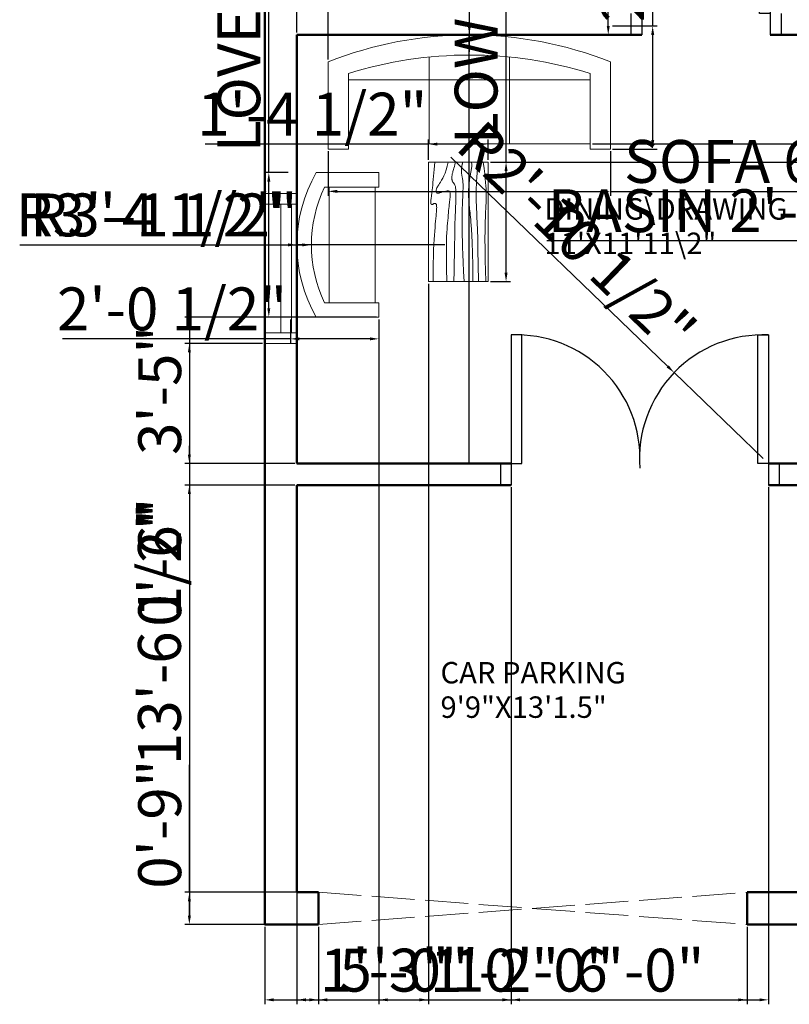
# Model space of a CAD drawing. Units: inches. Extents: x 3705 to 4206, y -1241 to -584.
# Tile 1 of 3: x 3705 to 3921, y -1162 to -886. Entities that reach past the tile are written whole.
import ezdxf

# ---------------------------------------------------------------- set-up
doc = ezdxf.new("R2010")
doc.units = ezdxf.units.IN
doc.linetypes.add('ACAD_ISO02W100', pattern=[15, 12, -3])
for name, color, linetype, lineweight in [('A-ANNO-DIMS', 2, 'Continuous', 18), ('A-AREA-IDEN', 7, 'Continuous', 25), ('A-DOOR', 3, 'Continuous', 25), ('A-DOOR-HIDN', 3, 'ACAD_ISO02W100', 18), ('A-FURN', 8, 'Continuous', 18), ('A-GLAZ', 4, 'Continuous', 18), ('A-WALL', 7, 'Continuous', 50)]:
    doc.layers.add(name, color=color, linetype=linetype, lineweight=lineweight)
doc.styles.get("Standard").update_dxf_attribs({"font": 'arial.ttf'})
doc.dimstyles.new('ISO-25', dxfattribs={"dimtxt": 12, "dimasz": 2.5, "dimexe": 1.25, "dimexo": 0.625, "dimtad": 1, "dimdec": 1, "dimlunit": 3, "dimtxsty": 'Standard', "dimcen": 2.5, "dimadec": 0, "dimazin": 0, "dimtfac": 1, "dimtdec": 1, "dimtmove": 0, "dimatfit": 3, "dimfxl": 1, "dimarcsym": 0})

# ---------------------------------------------------------------- blocks, each defined once
blk = doc.blocks.new('Sofa - Roundback Loveseat 5 ft.')
for p, q in [((0, -32.44198), (0, -5.99998)), ((-24, -33.99998), (-24, -11.46958)), ((24.00004, -33.99998), (24.00004, -11.46958)), ((-23.9998, -13.38178), (23.99986, -13.38178)), ((-24, -32.44198), (24.00004, -32.44198))]:
    blk.add_line(p, q)
for points in [[(-24, -33.99998), (-30, -33.99998), (-30, -7.99998)], [(30.00004, -7.99998), (30.00004, -33.99998), (24.00004, -33.99998)]]:
    blk.add_lwpolyline(points)
for centre, radius, start, end in [((0, -60.24998), 60.24998, 60.13715, 119.8628), ((0, -61.38438), 55.38444, 64.32083, 115.6792)]:
    blk.add_arc(centre, radius, start, end)
blk = doc.blocks.new('Sofa - Roundback 7 ft.')
for p, q in [((-12.00002, -32.4421), (-12.00003, -6.5971)), ((11.99997, -32.4421), (11.99998, -6.5971)), ((-36.000027, -34), (-36.000027, -11.4696)), ((35.99998, -34), (35.99998, -11.4696)), ((-35.999844, -13.3819), (35.9998, -13.3819)), ((-36.000027, -32.4421), (35.99998, -32.4421))]:
    blk.add_line(p, q)
for points in [[(-36.000027, -34), (-42.000027, -34), (-42.000027, -8)], [(41.99998, -8), (41.99998, -34), (35.99998, -34)]]:
    blk.add_lwpolyline(points)
for centre, radius, start, end in [((0, -114.25), 114.25, 68.43141, 111.5686), ((-0.00001, -127.1968), 121.1968, 72.72033, 107.2797)]:
    blk.add_arc(centre, radius, start, end)
blk = doc.blocks.new('Table - Rectangular Woodgrain 60 x 30 in.')
for p, q in [((0, 0), (0, -30)), ((60, 0), (0, 0)), ((60, -30), (60, 0)), ((0, -30), (60, -30))]:
    blk.add_line(p, q)
for points in [[(0, -2.4), (4.8155, -2.418), (9.0302, -2.4688), (12.709, -2.5477), (15.9167, -2.65), (18.7181, -2.7711), (21.1781, -2.9063), (23.3616, -3.0508), (25.3333, -3.2), (27.1477, -3.3495), (28.8172, -3.4958), (30.3437, -3.636), (31.7291, -3.7667), (32.9756, -3.8849), (34.0849, -3.9875), (35.059, -4.0714), (35.9, -4.1334), (36.6114, -4.1711), (37.2041, -4.1854), (37.6906, -4.1779), (38.0833, -4.15), (38.3948, -4.1034), (38.6375, -4.0396), (38.8239, -3.9602), (38.9666, -3.8667), (39.0764, -3.7608), (39.1573, -3.6448), (39.2116, -3.521), (39.2416, -3.3917), (39.2498, -3.2593), (39.2385, -3.1261), (39.21, -2.9944), (39.1666, -2.8667), (39.111, -2.7447), (39.0468, -2.6281), (38.978, -2.5163), (38.9083, -2.4083), (38.8418, -2.3035), (38.7823, -2.201), (38.7337, -2.1001), (38.7, -2), (38.6844, -1.9003), (38.6875, -1.8021), (38.7094, -1.707), (38.75, -1.6167), (38.8094, -1.5326), (38.8875, -1.4563), (38.9844, -1.3893), (39.1, -1.3333), (39.2351, -1.2896), (39.3937, -1.2583), (39.5804, -1.2396), (39.8, -1.2333), (40.057, -1.2396), (40.3562, -1.2583), (40.7023, -1.2896), (41.1, -1.3333), (41.5547, -1.3895), (42.0755, -1.4573), (42.6721, -1.5361), (43.3542, -1.625), (44.1316, -1.7233), (45.014, -1.8302), (46.0114, -1.9449), (47.1333, -2.0667), (48.3862, -2.1947), (49.7625, -2.3281), (51.2513, -2.4663), (52.8416, -2.6083), (54.5226, -2.7535), (56.2833, -2.9011), (58.1127, -3.0501), (60, -3.2)], [(0, -9.2), (6.5759, -9.0858), (11.9385, -9.0365), (16.2527, -9.0418), (19.6833, -9.0917), (22.3952, -9.1759), (24.5531, -9.2844), (26.322, -9.4069), (27.8666, -9.5333), (29.3241, -9.6553), (30.7203, -9.7719), (32.0532, -9.8837), (33.3208, -9.9917), (34.5213, -10.0965), (35.6526, -10.199), (36.7128, -10.2999), (37.7, -10.4), (38.6129, -10.4996), (39.4531, -10.5969), (40.223, -10.6895), (40.925, -10.775), (41.5613, -10.8512), (42.1344, -10.9156), (42.6465, -10.966), (43.1, -11), (43.4976, -11.0158), (43.8437, -11.0136), (44.143, -10.9942), (44.4, -10.9583), (44.6195, -10.9069), (44.8062, -10.8406), (44.9648, -10.7603), (45.1, -10.6667), (45.2155, -10.5598), (45.3114, -10.4365), (45.3871, -10.2929), (45.4416, -10.125), (45.4743, -9.929), (45.4844, -9.7011), (45.4709, -9.4371), (45.4333, -9.1333), (45.3716, -8.7883), (45.2896, -8.4104), (45.1919, -8.0107), (45.0833, -7.6), (44.9685, -7.1893), (44.8521, -6.7896), (44.7388, -6.4117), (44.6333, -6.0667), (44.54, -5.7628), (44.4614, -5.4979), (44.4001, -5.2675), (44.3583, -5.0667), (44.3384, -4.8909), (44.3427, -4.7354), (44.3736, -4.5956), (44.4333, -4.4667), (44.5236, -4.3453), (44.6427, -4.2333), (44.7884, -4.1339), (44.9583, -4.05), (45.1501, -3.9849), (45.3614, -3.9417), (45.59, -3.9234), (45.8333, -3.9333), (46.0915, -3.9749), (46.3734, -4.0531), (46.6906, -4.1736), (47.0542, -4.3417), (47.4756, -4.5629), (47.9661, -4.8427), (48.5372, -5.1866), (49.2, -5.6), (49.9676, -6.0844), (50.8594, -6.625), (51.8965, -7.2031), (53.1, -7.8), (54.491, -8.3969), (56.0906, -8.975), (57.9199, -9.5156), (60, -10)], [(0, -12.8), (5.1847, -12.9322), (9.6213, -13.0323), (13.3963, -13.1059), (16.5958, -13.1583), (19.3063, -13.1952), (21.614, -13.2219), (23.6054, -13.2439), (25.3666, -13.2667), (26.9728, -13.2947), (28.4531, -13.3281), (29.8256, -13.3663), (31.1083, -13.4083), (32.3191, -13.4535), (33.476, -13.501), (34.597, -13.5501), (35.7, -13.6), (36.7984, -13.6497), (37.8875, -13.6979), (38.9578, -13.743), (40, -13.7833), (41.0047, -13.8174), (41.9625, -13.8438), (42.864, -13.8607), (43.7, -13.8667), (44.4631, -13.8604), (45.1552, -13.8417), (45.7801, -13.8104), (46.3416, -13.7667), (46.8439, -13.7104), (47.2906, -13.6417), (47.6858, -13.5604), (48.0333, -13.4667), (48.3375, -13.3608), (48.6042, -13.2448), (48.8396, -13.121), (49.05, -12.9917), (49.2417, -12.8593), (49.4208, -12.7261), (49.5937, -12.5944), (49.7667, -12.4667), (49.9452, -12.3451), (50.1323, -12.2313), (50.3303, -12.1268), (50.5416, -12.0333), (50.7686, -11.9524), (51.0135, -11.8854), (51.2788, -11.8341), (51.5666, -11.8), (51.8785, -11.7843), (52.2116, -11.7865), (52.562, -11.8059), (52.926, -11.8417), (53.2998, -11.8931), (53.6795, -11.9594), (54.0614, -12.0397), (54.4416, -12.1333), (54.8223, -12.2401), (55.2293, -12.3625), (55.6942, -12.5037), (56.2489, -12.6667), (56.9251, -12.8547), (57.7545, -13.0708), (58.7689, -13.3182), (60, -13.6)], [(0, -18), (5.124, -17.7273), (9.6609, -17.5057), (13.6705, -17.3303), (17.2125, -17.1958), (20.3467, -17.0973), (23.1328, -17.0297), (25.6307, -16.9878), (27.9, -16.9667), (29.9928, -16.9617), (31.9302, -16.9703), (33.7254, -16.9907), (35.3917, -17.0208), (36.9423, -17.0588), (38.3906, -17.1026), (39.7499, -17.1503), (41.0333, -17.2), (42.2519, -17.2496), (43.4073, -17.2969), (44.4986, -17.3395), (45.525, -17.375), (46.4858, -17.4012), (47.3802, -17.4156), (48.2074, -17.416), (48.9667, -17.4), (49.6583, -17.3662), (50.2872, -17.3167), (50.8595, -17.2547), (51.3812, -17.1833), (51.8584, -17.1057), (52.2971, -17.025), (52.7034, -16.9443), (53.0833, -16.8667), (53.443, -16.7951), (53.789, -16.7313), (54.128, -16.6768), (54.4666, -16.6334), (54.8115, -16.6024), (55.1693, -16.5854), (55.5465, -16.5841), (55.95, -16.6), (56.3828, -16.6337), (56.8346, -16.6823), (57.2915, -16.7418), (57.7396, -16.8084), (58.165, -16.878), (58.5539, -16.9469), (58.8924, -17.0111), (59.1666, -17.0667), (59.3679, -17.1107), (59.5078, -17.1438), (59.6032, -17.1675), (59.6708, -17.1833), (59.7275, -17.193), (59.7901, -17.1979), (59.8753, -17.1998), (60, -17.2)], [(0, -22.4), (8.0098, -22.2501), (14.4094, -22.1011), (19.4168, -21.9535), (23.25, -21.8083), (26.1269, -21.6663), (28.2656, -21.5281), (29.884, -21.3947), (31.2, -21.2667), (32.3967, -21.1448), (33.5172, -21.0292), (34.5697, -20.9198), (35.5625, -20.8167), (36.5037, -20.7198), (37.4015, -20.6292), (38.2642, -20.5448), (39.1, -20.4667), (39.9164, -20.3951), (40.7187, -20.3313), (41.5117, -20.2768), (42.3, -20.2333), (43.0883, -20.2024), (43.8812, -20.1854), (44.6836, -20.1841), (45.5, -20.2), (46.3328, -20.234), (47.1747, -20.2844), (48.0163, -20.3488), (48.8479, -20.425), (49.66, -20.5106), (50.4429, -20.6031), (51.1872, -20.7004), (51.8833, -20.8), (52.5246, -20.8999), (53.1166, -20.9995), (53.6681, -21.0983), (54.1875, -21.1958), (54.6834, -21.2919), (55.1646, -21.3859), (55.6394, -21.4777), (56.1167, -21.5667), (56.6028, -21.6515), (57.0961, -21.7266), (57.5929, -21.7852), (58.0896, -21.8208), (58.5823, -21.8268), (59.0674, -21.7964), (59.5412, -21.723), (60, -21.6)], [(0, -25.2), (8.6355, -25.0504), (15.7026, -24.9031), (21.4049, -24.7606), (25.9458, -24.625), (29.529, -24.4988), (32.3578, -24.3844), (34.6359, -24.284), (36.5667, -24.2), (38.3213, -24.1341), (39.9417, -24.0854), (41.437, -24.0523), (42.8167, -24.0333), (44.0901, -24.0268), (45.2667, -24.0313), (46.3557, -24.0451), (47.3667, -24.0667), (48.309, -24.0947), (49.1928, -24.1287), (50.0284, -24.168), (50.826, -24.2125), (51.5959, -24.2617), (52.3483, -24.3151), (53.0935, -24.3725), (53.8417, -24.4334), (54.6009, -24.497), (55.3699, -24.561), (56.1454, -24.6226), (56.9239, -24.6792), (57.7021, -24.7279), (58.4764, -24.7662), (59.2435, -24.7911), (60, -24.8)], [(0, -28.8), (5.6867, -28.6681), (10.45, -28.5698), (14.407, -28.5012), (17.675, -28.4584), (20.3711, -28.4374), (22.6125, -28.4344), (24.5164, -28.4455), (26.2, -28.4667), (27.762, -28.4947), (29.2276, -28.5281), (30.6033, -28.5663), (31.8958, -28.6084), (33.1118, -28.6535), (34.2578, -28.7011), (35.3405, -28.7501), (36.3666, -28.8), (37.3443, -28.8497), (38.288, -28.8974), (39.2137, -28.9412), (40.1375, -28.9792), (41.0753, -29.0093), (42.0432, -29.0297), (43.0572, -29.0384), (44.1333, -29.0333), (45.2936, -29.0114), (46.5843, -28.9641), (48.0579, -28.8816), (49.7666, -28.7542), (51.7629, -28.5721), (54.0989, -28.3255), (56.8272, -28.0048), (60, -27.6)]]:
    blk.add_lwpolyline(points)
blk = doc.blocks.new('DOOR-SINGLE-36IN')
for p, q in [((0, 6), (0, 0)), ((3, 6), (3, 0)), ((39, 6), (39, 0)), ((42, 6), (42, 0))]:
    blk.add_line(p, q)
blk.add_lwpolyline([(39, 6), (36, 6), (36, 42), (39, 42)], close=True)
blk.add_arc((37.5, 7.5), 34.53, 87.5104, 182.4896)
blk = doc.blocks.new('WIN-SASH-36IN')
for p, q in [((0, 9), (0, 0)), ((36, 0), (36, 9)), ((0, 4.5), (36, 4.5)), ((0, 1.5), (36, 1.5)), ((0, 1.5), (36, 1.5))]:
    blk.add_line(p, q)
blk = doc.blocks.new('*D21')
at = {"layer": 'A-ANNO-DIMS', "color": 0, "lineweight": -2, "transparency": 16777216}
for p, q in [((3870.22, -848.33), (3870.22, -651.86)), ((3875.95, -848.33), (3868.97, -848.33)), ((3870.22, -888.25), (3870.22, -850.83)), ((3875.95, -890.75), (3868.97, -890.75))]:
    blk.add_line(p, q, dxfattribs=at)
at = {"layer": 'A-ANNO-DIMS', "color": 0, "transparency": 16777216}
for points in [[(3869.8, -850.83), (3870.63, -850.83), (3870.22, -848.33)], [(3869.8, -888.25), (3870.63, -888.25), (3870.22, -890.75)]]:
    blk.add_solid(points, dxfattribs=at)
at = {"layer": 'Defpoints', "color": 0, "transparency": 16777216}
for p in [(3870.22, -848.33), (3876.58, -848.33), (3876.58, -890.75)]:
    blk.add_point(p, dxfattribs=at)
at = {"layer": 'A-ANNO-DIMS', "color": 0, "transparency": 16777216, "insert": (3863.38, -748.84), "char_height": 12, "attachment_point": 5, "rotation": 90}
blk.add_mtext('DOOR SET 3\'-6 1/2" TYP.', dxfattribs=at)
blk = doc.blocks.new('*D23')
at = {"layer": 'A-ANNO-DIMS', "color": 0, "lineweight": -2, "transparency": 16777216}
for p, q in [((3775.21, -929.3), (3775.21, -773.05)), ((3780.66, -929.3), (3773.96, -929.3)), ((3775.21, -967.26), (3775.21, -931.8)), ((3780.66, -969.76), (3773.96, -969.76))]:
    blk.add_line(p, q, dxfattribs=at)
at = {"layer": 'A-ANNO-DIMS', "color": 0, "transparency": 16777216}
for points in [[(3774.79, -931.8), (3775.63, -931.8), (3775.21, -929.3)], [(3774.79, -967.26), (3775.63, -967.26), (3775.21, -969.76)]]:
    blk.add_solid(points, dxfattribs=at)
at = {"layer": 'Defpoints', "color": 0, "transparency": 16777216}
for p in [(3775.21, -929.3), (3781.28, -929.3), (3781.28, -969.76)]:
    blk.add_point(p, dxfattribs=at)
at = {"layer": 'A-ANNO-DIMS', "color": 0, "transparency": 16777216, "insert": (3768.37, -849.92), "char_height": 12, "attachment_point": 5, "rotation": 90}
blk.add_mtext('LOVESEAT 3\'-4 1/2"', dxfattribs=at)
blk = doc.blocks.new('*D24')
at = {"layer": 'A-ANNO-DIMS', "color": 0, "lineweight": -2, "transparency": 16777216}
for p, q in [((3781.28, -970.39), (3781.28, -977.08)), ((3806.01, -970.39), (3806.01, -977.08)), ((3781.28, -975.83), (3717.47, -975.83)), ((3803.51, -975.83), (3783.78, -975.83))]:
    blk.add_line(p, q, dxfattribs=at)
at = {"layer": 'A-ANNO-DIMS', "color": 0, "transparency": 16777216}
for points in [[(3783.78, -975.42), (3783.78, -976.25), (3781.28, -975.83)], [(3803.51, -975.42), (3803.51, -976.25), (3806.01, -975.83)]]:
    blk.add_solid(points, dxfattribs=at)
at = {"layer": 'Defpoints', "color": 0, "transparency": 16777216}
for p in [(3781.28, -969.76), (3806.01, -969.76), (3781.28, -975.83)]:
    blk.add_point(p, dxfattribs=at)
at = {"layer": 'A-ANNO-DIMS', "color": 0, "transparency": 16777216, "insert": (3748.12, -969), "char_height": 12, "attachment_point": 5}
blk.add_mtext('2\'-0 1/2"', dxfattribs=at)
blk = doc.blocks.new('*D25')
at = {"layer": 'A-ANNO-DIMS', "color": 0, "lineweight": -2, "transparency": 16777216}
for p, q in [((3791.85, -923.33), (3791.85, -935.8)), ((3870.81, -923.33), (3870.81, -935.8)), ((3794.35, -934.55), (3868.31, -934.55)), ((3870.81, -934.55), (3956.7, -934.55))]:
    blk.add_line(p, q, dxfattribs=at)
at = {"layer": 'A-ANNO-DIMS', "color": 0, "transparency": 16777216}
for points in [[(3794.35, -934.13), (3794.35, -934.97), (3791.85, -934.55)], [(3868.31, -934.13), (3868.31, -934.97), (3870.81, -934.55)]]:
    blk.add_solid(points, dxfattribs=at)
at = {"layer": 'Defpoints', "color": 0, "transparency": 16777216}
for p in [(3791.85, -922.71), (3870.81, -922.71), (3870.81, -934.55)]:
    blk.add_point(p, dxfattribs=at)
at = {"layer": 'A-ANNO-DIMS', "color": 0, "transparency": 16777216, "insert": (3915, -927.72), "char_height": 12, "attachment_point": 5}
blk.add_mtext('SOFA 6\'-7"', dxfattribs=at)
blk = doc.blocks.new('*D26')
at = {"layer": 'A-ANNO-DIMS', "color": 0, "lineweight": -2, "transparency": 16777216}
for p, q in [((3882.65, -888.24), (3882.65, -815.1)), ((3871.43, -888.24), (3883.9, -888.24)), ((3882.65, -920.21), (3882.65, -890.74)), ((3871.43, -922.71), (3883.9, -922.71))]:
    blk.add_line(p, q, dxfattribs=at)
at = {"layer": 'A-ANNO-DIMS', "color": 0, "transparency": 16777216}
for points in [[(3882.23, -890.74), (3883.07, -890.74), (3882.65, -888.24)], [(3882.23, -920.21), (3883.07, -920.21), (3882.65, -922.71)]]:
    blk.add_solid(points, dxfattribs=at)
at = {"layer": 'Defpoints', "color": 0, "transparency": 16777216}
for p in [(3870.81, -888.24), (3882.65, -888.24), (3870.81, -922.71)]:
    blk.add_point(p, dxfattribs=at)
at = {"layer": 'A-ANNO-DIMS', "color": 0, "transparency": 16777216, "insert": (3875.82, -850.42), "char_height": 12, "attachment_point": 5, "rotation": 90}
blk.add_mtext('2\'-10 1/2"', dxfattribs=at)
blk = doc.blocks.new('*D27')
at = {"layer": 'A-ANNO-DIMS', "color": 0, "lineweight": -2, "transparency": 16777216}
for p, q in [((3841.61, -926.33), (3841.61, -762.65)), ((3837.22, -926.33), (3842.86, -926.33)), ((3841.61, -957.3), (3841.61, -928.83)), ((3837.22, -959.8), (3842.86, -959.8))]:
    blk.add_line(p, q, dxfattribs=at)
at = {"layer": 'A-ANNO-DIMS', "color": 0, "transparency": 16777216}
for points in [[(3841.2, -928.83), (3842.03, -928.83), (3841.61, -926.33)], [(3841.2, -957.3), (3842.03, -957.3), (3841.61, -959.8)]]:
    blk.add_solid(points, dxfattribs=at)
at = {"layer": 'Defpoints', "color": 0, "transparency": 16777216}
for p in [(3836.59, -926.33), (3841.61, -926.33), (3836.59, -959.8)]:
    blk.add_point(p, dxfattribs=at)
at = {"layer": 'A-ANNO-DIMS', "color": 0, "transparency": 16777216, "insert": (3834.78, -843.24), "char_height": 12, "attachment_point": 5, "rotation": 90}
blk.add_mtext('LOW TABLE 2\'-9 1/2"', dxfattribs=at)
blk = doc.blocks.new('*D28')
at = {"layer": 'A-ANNO-DIMS', "color": 0, "lineweight": -2, "transparency": 16777216}
for p, q in [((3819.86, -925.71), (3819.86, -920.07)), ((3836.59, -925.71), (3836.59, -920.07)), ((3819.86, -921.32), (3757.38, -921.32)), ((3834.09, -921.32), (3822.36, -921.32))]:
    blk.add_line(p, q, dxfattribs=at)
at = {"layer": 'A-ANNO-DIMS', "color": 0, "transparency": 16777216}
for points in [[(3822.36, -920.9), (3822.36, -921.73), (3819.86, -921.32)], [(3834.09, -920.9), (3834.09, -921.73), (3836.59, -921.32)]]:
    blk.add_solid(points, dxfattribs=at)
at = {"layer": 'Defpoints', "color": 0, "transparency": 16777216}
for p in [(3819.86, -921.32), (3819.86, -926.33), (3836.59, -926.33)]:
    blk.add_point(p, dxfattribs=at)
at = {"layer": 'A-ANNO-DIMS', "color": 0, "transparency": 16777216, "insert": (3787.37, -914.49), "char_height": 12, "attachment_point": 5}
blk.add_mtext('1\'-4 1/2"', dxfattribs=at)
blk = doc.blocks.new('*D31')
at = {"layer": 'A-ANNO-DIMS', "color": 0, "lineweight": -2, "transparency": 16777216}
for p, q in [((3943.08, -945.37), (3943.08, -949.6)), ((3967.08, -945.37), (3967.08, -949.6)), ((3943.08, -948.35), (3853, -948.35)), ((3964.58, -948.35), (3945.58, -948.35))]:
    blk.add_line(p, q, dxfattribs=at)
at = {"layer": 'A-ANNO-DIMS', "color": 0, "transparency": 16777216}
for points in [[(3945.58, -947.93), (3945.58, -948.76), (3943.08, -948.35)], [(3964.58, -947.93), (3964.58, -948.76), (3967.08, -948.35)]]:
    blk.add_solid(points, dxfattribs=at)
at = {"layer": 'Defpoints', "color": 0, "transparency": 16777216}
for p in [(3943.08, -944.75), (3967.08, -944.75), (3943.08, -948.35)]:
    blk.add_point(p, dxfattribs=at)
at = {"layer": 'A-ANNO-DIMS', "color": 0, "transparency": 16777216, "insert": (3896.79, -941.52), "char_height": 12, "attachment_point": 5}
blk.add_mtext('BASIN 2\'-0"', dxfattribs=at)
blk = doc.blocks.new('*D39')
at = {"layer": 'A-ANNO-DIMS', "color": 0, "lineweight": -2, "transparency": 16777216}
for p, q in [((3773.45, -977.11), (3751.73, -977.11)), ((3752.98, -979.61), (3752.98, -1137.25)), ((3773.45, -1139.75), (3751.73, -1139.75))]:
    blk.add_line(p, q, dxfattribs=at)
at = {"layer": 'A-ANNO-DIMS', "color": 0, "transparency": 16777216}
for points in [[(3752.56, -979.61), (3753.4, -979.61), (3752.98, -977.11)], [(3752.56, -1137.25), (3753.4, -1137.25), (3752.98, -1139.75)]]:
    blk.add_solid(points, dxfattribs=at)
at = {"layer": 'Defpoints', "color": 0, "transparency": 16777216}
for p in [(3774.08, -977.11), (3752.98, -1139.75), (3774.08, -1139.75)]:
    blk.add_point(p, dxfattribs=at)
at = {"layer": 'A-ANNO-DIMS', "color": 0, "transparency": 16777216, "insert": (3746.15, -1058.43), "char_height": 12, "attachment_point": 5, "rotation": 90}
blk.add_mtext('13\'-6 1/2"', dxfattribs=at)
blk = doc.blocks.new('*D43')
at = {"layer": 'A-ANNO-DIMS', "color": 0, "lineweight": -2, "transparency": 16777216}
for p, q in [((3789.08, -1140.37), (3789.08, -1162.1)), ((3909.08, -1140.37), (3909.08, -1162.1)), ((3791.58, -1160.85), (3906.58, -1160.85))]:
    blk.add_line(p, q, dxfattribs=at)
at = {"layer": 'A-ANNO-DIMS', "color": 0, "transparency": 16777216}
for points in [[(3791.58, -1160.43), (3791.58, -1161.26), (3789.08, -1160.85)], [(3906.58, -1160.43), (3906.58, -1161.26), (3909.08, -1160.85)]]:
    blk.add_solid(points, dxfattribs=at)
at = {"layer": 'Defpoints', "color": 0, "transparency": 16777216}
for p in [(3789.08, -1139.75), (3909.08, -1139.75), (3909.08, -1160.85)]:
    blk.add_point(p, dxfattribs=at)
at = {"layer": 'A-ANNO-DIMS', "color": 0, "transparency": 16777216, "insert": (3849.08, -1154.1), "char_height": 12, "attachment_point": 5}
blk.add_mtext('10\'-0"', dxfattribs=at)
blk = doc.blocks.new('*D44')
at = {"layer": 'A-ANNO-DIMS', "color": 0, "lineweight": -2, "transparency": 16777216}
for p, q in [((3774.08, -1140.37), (3774.08, -1162.1)), ((3789.08, -1140.37), (3789.08, -1162.1)), ((3776.58, -1160.85), (3786.58, -1160.85)), ((3789.08, -1160.85), (3823.6, -1160.85))]:
    blk.add_line(p, q, dxfattribs=at)
at = {"layer": 'A-ANNO-DIMS', "color": 0, "transparency": 16777216}
for points in [[(3776.58, -1160.43), (3776.58, -1161.26), (3774.08, -1160.85)], [(3786.58, -1160.43), (3786.58, -1161.26), (3789.08, -1160.85)]]:
    blk.add_solid(points, dxfattribs=at)
at = {"layer": 'Defpoints', "color": 0, "transparency": 16777216}
for p in [(3774.08, -1139.75), (3789.08, -1139.75), (3789.08, -1160.85)]:
    blk.add_point(p, dxfattribs=at)
at = {"layer": 'A-ANNO-DIMS', "color": 0, "transparency": 16777216, "insert": (3807.59, -1154.09), "char_height": 12, "attachment_point": 5}
blk.add_mtext('1\'-3"', dxfattribs=at)
blk = doc.blocks.new('*D47')
at = {"layer": 'A-ANNO-DIMS', "color": 0, "lineweight": -2, "transparency": 16777216}
for p, q in [((3843.06, -1017.37), (3843.06, -1162.1)), ((3915.06, -1017.37), (3915.06, -1162.1)), ((3845.56, -1160.85), (3912.56, -1160.85))]:
    blk.add_line(p, q, dxfattribs=at)
at = {"layer": 'A-ANNO-DIMS', "color": 0, "transparency": 16777216}
for points in [[(3845.56, -1160.43), (3845.56, -1161.26), (3843.06, -1160.85)], [(3912.56, -1160.43), (3912.56, -1161.26), (3915.06, -1160.85)]]:
    blk.add_solid(points, dxfattribs=at)
at = {"layer": 'Defpoints', "color": 0, "transparency": 16777216}
for p in [(3843.06, -1016.75), (3915.06, -1016.75), (3915.06, -1160.85)]:
    blk.add_point(p, dxfattribs=at)
at = {"layer": 'A-ANNO-DIMS', "color": 0, "transparency": 16777216, "insert": (3879.06, -1154.1), "char_height": 12, "attachment_point": 5}
blk.add_mtext('6\'-0"', dxfattribs=at)
blk = doc.blocks.new('*D48')
at = {"layer": 'A-ANNO-DIMS', "color": 0, "lineweight": -2, "transparency": 16777216}
for p, q in [((3783.08, -1017.37), (3783.08, -1162.1)), ((3843.06, -1017.37), (3843.06, -1162.1)), ((3785.58, -1160.85), (3840.56, -1160.85))]:
    blk.add_line(p, q, dxfattribs=at)
at = {"layer": 'A-ANNO-DIMS', "color": 0, "transparency": 16777216}
for points in [[(3785.58, -1160.43), (3785.58, -1161.26), (3783.08, -1160.85)], [(3840.56, -1160.43), (3840.56, -1161.26), (3843.06, -1160.85)]]:
    blk.add_solid(points, dxfattribs=at)
at = {"layer": 'Defpoints', "color": 0, "transparency": 16777216}
for p in [(3783.08, -1016.75), (3843.06, -1016.75), (3843.06, -1160.85)]:
    blk.add_point(p, dxfattribs=at)
at = {"layer": 'A-ANNO-DIMS', "color": 0, "transparency": 16777216, "insert": (3813.07, -1154.1), "char_height": 12, "attachment_point": 5}
blk.add_mtext('5\'-0"', dxfattribs=at)
blk = doc.blocks.new('*D49')
at = {"layer": 'A-ANNO-DIMS', "color": 0, "lineweight": -2, "transparency": 16777216}
for p, q in [((3752.98, -1130.75), (3752.98, -1095.1)), ((3788.45, -1130.75), (3751.73, -1130.75)), ((3752.98, -1137.25), (3752.98, -1133.25)), ((3788.45, -1139.75), (3751.73, -1139.75))]:
    blk.add_line(p, q, dxfattribs=at)
at = {"layer": 'A-ANNO-DIMS', "color": 0, "transparency": 16777216}
for points in [[(3752.56, -1133.25), (3753.4, -1133.25), (3752.98, -1130.75)], [(3752.56, -1137.25), (3753.4, -1137.25), (3752.98, -1139.75)]]:
    blk.add_solid(points, dxfattribs=at)
at = {"layer": 'Defpoints', "color": 0, "transparency": 16777216}
for p in [(3752.98, -1130.75), (3789.08, -1130.75), (3789.08, -1139.75)]:
    blk.add_point(p, dxfattribs=at)
at = {"layer": 'A-ANNO-DIMS', "color": 0, "transparency": 16777216, "insert": (3746.23, -1111.67), "char_height": 12, "attachment_point": 5, "rotation": 90}
blk.add_mtext('0\'-9"', dxfattribs=at)
blk = doc.blocks.new('*D50')
at = {"layer": 'A-ANNO-DIMS', "color": 0, "lineweight": -2, "transparency": 16777216}
for p, q in [((3752.98, -1008.25), (3752.98, -1005.75)), ((3782.45, -1010.75), (3751.73, -1010.75)), ((3752.98, -1010.75), (3752.98, -1016.75)), ((3782.45, -1016.75), (3751.73, -1016.75)), ((3752.98, -1019.25), (3752.98, -1054.9))]:
    blk.add_line(p, q, dxfattribs=at)
at = {"layer": 'A-ANNO-DIMS', "color": 0, "transparency": 16777216}
for points in [[(3752.56, -1008.25), (3753.4, -1008.25), (3752.98, -1010.75)], [(3752.56, -1019.25), (3753.4, -1019.25), (3752.98, -1016.75)]]:
    blk.add_solid(points, dxfattribs=at)
at = {"layer": 'Defpoints', "color": 0, "transparency": 16777216}
for p in [(3783.08, -1010.75), (3752.98, -1016.75), (3783.08, -1016.75)]:
    blk.add_point(p, dxfattribs=at)
at = {"layer": 'A-ANNO-DIMS', "color": 0, "transparency": 16777216, "insert": (3746.23, -1038.32), "char_height": 12, "attachment_point": 5, "rotation": 90}
blk.add_mtext('0\'-6"', dxfattribs=at)
blk = doc.blocks.new('*D56')
at = {"layer": 'A-ANNO-DIMS', "color": 0, "lineweight": -2, "transparency": 16777216}
for p, q in [((3783.08, -890.12), (3783.08, -733.4)), ((3785.58, -734.65), (3789.35, -734.65)), ((3791.85, -897.64), (3791.85, -733.4)), ((3791.85, -734.65), (3827.5, -734.65))]:
    blk.add_line(p, q, dxfattribs=at)
at = {"layer": 'A-ANNO-DIMS', "color": 0, "transparency": 16777216}
for points in [[(3785.58, -734.23), (3785.58, -735.06), (3783.08, -734.65)], [(3789.35, -734.23), (3789.35, -735.06), (3791.85, -734.65)]]:
    blk.add_solid(points, dxfattribs=at)
at = {"layer": 'Defpoints', "color": 0, "transparency": 16777216}
for p in [(3791.85, -734.65), (3783.08, -890.75), (3791.85, -898.27)]:
    blk.add_point(p, dxfattribs=at)
at = {"layer": 'A-ANNO-DIMS', "color": 0, "transparency": 16777216, "insert": (3810.93, -727.9), "char_height": 12, "attachment_point": 5}
blk.add_mtext('0\'-9"', dxfattribs=at)
blk = doc.blocks.new('*D57')
at = {"layer": 'A-ANNO-DIMS', "color": 0, "lineweight": -2, "transparency": 16777216}
for p, q in [((3819.86, -960.42), (3819.86, -1162.1)), ((3806.01, -970.39), (3806.01, -1162.1)), ((3808.51, -1160.85), (3817.36, -1160.85)), ((3819.86, -1160.85), (3854.38, -1160.85))]:
    blk.add_line(p, q, dxfattribs=at)
at = {"layer": 'A-ANNO-DIMS', "color": 0, "transparency": 16777216}
for points in [[(3808.51, -1160.43), (3808.51, -1161.26), (3806.01, -1160.85)], [(3817.36, -1160.43), (3817.36, -1161.26), (3819.86, -1160.85)]]:
    blk.add_solid(points, dxfattribs=at)
at = {"layer": 'Defpoints', "color": 0, "transparency": 16777216}
for p in [(3819.86, -959.8), (3806.01, -969.76), (3819.86, -1160.85)]:
    blk.add_point(p, dxfattribs=at)
at = {"layer": 'A-ANNO-DIMS', "color": 0, "transparency": 16777216, "insert": (3838.37, -1154.2), "char_height": 12, "attachment_point": 5}
blk.add_mtext('1\'-2"', dxfattribs=at)
blk = doc.blocks.new('*D58')
at = {"layer": 'A-ANNO-DIMS', "color": 0, "lineweight": -2, "transparency": 16777216}
for p, q in [((3805.39, -969.76), (3751.73, -969.76)), ((3752.98, -972.26), (3752.98, -1008.25)), ((3782.45, -1010.75), (3751.73, -1010.75))]:
    blk.add_line(p, q, dxfattribs=at)
at = {"layer": 'A-ANNO-DIMS', "color": 0, "transparency": 16777216}
for points in [[(3752.56, -972.26), (3753.4, -972.26), (3752.98, -969.76)], [(3752.56, -1008.25), (3753.4, -1008.25), (3752.98, -1010.75)]]:
    blk.add_solid(points, dxfattribs=at)
at = {"layer": 'Defpoints', "color": 0, "transparency": 16777216}
for p in [(3806.01, -969.76), (3752.98, -1010.75), (3783.08, -1010.75)]:
    blk.add_point(p, dxfattribs=at)
at = {"layer": 'A-ANNO-DIMS', "color": 0, "transparency": 16777216, "insert": (3746.22, -990.26), "char_height": 12, "attachment_point": 5, "rotation": 90}
blk.add_mtext('3\'-5"', dxfattribs=at)
blk = doc.blocks.new('*D59')
at = {"layer": 'A-ANNO-DIMS', "color": 0, "lineweight": -2, "transparency": 16777216}
for p, q in [((4095.18, -918.74), (4095.18, -916.24)), ((3865.79, -921.24), (4096.43, -921.24)), ((4095.18, -921.24), (4095.18, -926.33)), ((3837.22, -926.33), (4096.43, -926.33)), ((4095.18, -928.83), (4095.18, -964.48))]:
    blk.add_line(p, q, dxfattribs=at)
at = {"layer": 'A-ANNO-DIMS', "color": 0, "transparency": 16777216}
for points in [[(4094.76, -918.74), (4095.6, -918.74), (4095.18, -921.24)], [(4094.76, -928.83), (4095.6, -928.83), (4095.18, -926.33)]]:
    blk.add_solid(points, dxfattribs=at)
at = {"layer": 'Defpoints', "color": 0, "transparency": 16777216}
for p in [(3865.17, -921.24), (3836.59, -926.33), (4095.18, -926.33)]:
    blk.add_point(p, dxfattribs=at)
at = {"layer": 'A-ANNO-DIMS', "color": 0, "transparency": 16777216, "insert": (4088.43, -947.91), "char_height": 12, "attachment_point": 5, "rotation": 90}
blk.add_mtext('0\'-5"', dxfattribs=at)
blk = doc.blocks.new('*D60')
at = {"layer": 'A-ANNO-DIMS', "color": 0, "lineweight": -2, "transparency": 16777216}
for p, q in [((3831.33, -805.72), (3831.33, -893.89)), ((3831.33, -1010.31), (3831.33, -896.39))]:
    blk.add_line(p, q, dxfattribs=at)
at = {"layer": 'A-ANNO-DIMS', "color": 0, "transparency": 16777216}
blk.add_solid([(3831.75, -893.89), (3830.91, -893.89), (3831.33, -896.39)], dxfattribs=at)
at = {"layer": 'Defpoints', "color": 0, "transparency": 16777216}
for p in [(3831.33, -896.39), (3831.33, -1010.31)]:
    blk.add_point(p, dxfattribs=at)
at = {"layer": 'A-ANNO-DIMS', "color": 0, "transparency": 16777216, "insert": (3838.08, -828.04), "char_height": 12, "attachment_point": 5, "rotation": 270.0001}
blk.add_mtext('R9\'-6"', dxfattribs=at)
blk = doc.blocks.new('*D61')
at = {"layer": 'A-ANNO-DIMS', "color": 0, "lineweight": -2, "transparency": 16777216}
for p, q in [((3831.33, -785.35), (3831.33, -888.25)), ((3831.33, -998.14), (3831.33, -890.75))]:
    blk.add_line(p, q, dxfattribs=at)
at = {"layer": 'A-ANNO-DIMS', "color": 0, "transparency": 16777216}
blk.add_solid([(3831.75, -888.25), (3830.91, -888.25), (3831.33, -890.75)], dxfattribs=at)
at = {"layer": 'Defpoints', "color": 0, "transparency": 16777216}
for p in [(3831.33, -890.75), (3831.33, -998.14)]:
    blk.add_point(p, dxfattribs=at)
at = {"layer": 'A-ANNO-DIMS', "color": 0, "transparency": 16777216, "insert": (3838.16, -826.31), "char_height": 12, "attachment_point": 5, "rotation": 270.0001}
blk.add_mtext('R8\'-11 1/2"', dxfattribs=at)
blk = doc.blocks.new('*D62')
at = {"layer": 'A-ANNO-DIMS', "color": 0, "lineweight": -2, "transparency": 16777216}
for p, q in [((3705.48, -949.53), (3780.58, -949.53)), ((3823.72, -949.53), (3783.08, -949.53))]:
    blk.add_line(p, q, dxfattribs=at)
at = {"layer": 'A-ANNO-DIMS', "color": 0, "transparency": 16777216}
blk.add_solid([(3780.58, -949.11), (3780.58, -949.95), (3783.08, -949.53)], dxfattribs=at)
at = {"layer": 'Defpoints', "color": 0, "transparency": 16777216}
for p in [(3783.08, -949.53), (3823.72, -949.53)]:
    blk.add_point(p, dxfattribs=at)
at = {"layer": 'A-ANNO-DIMS', "color": 0, "transparency": 16777216, "insert": (3741.78, -942.7), "char_height": 12, "attachment_point": 5, "rotation": 359.9994}
blk.add_mtext('R3\'-4 1/2"', dxfattribs=at)
blk = doc.blocks.new('*D63')
at = {"layer": 'A-ANNO-DIMS', "color": 0, "lineweight": -2, "transparency": 16777216}
for p, q in [((3709.53, -949.53), (3784.63, -949.53)), ((3824.48, -949.53), (3787.13, -949.53))]:
    blk.add_line(p, q, dxfattribs=at)
at = {"layer": 'A-ANNO-DIMS', "color": 0, "transparency": 16777216}
blk.add_solid([(3784.63, -949.11), (3784.63, -949.95), (3787.13, -949.53)], dxfattribs=at)
at = {"layer": 'Defpoints', "color": 0, "transparency": 16777216}
for p in [(3787.13, -949.53), (3824.48, -949.53)]:
    blk.add_point(p, dxfattribs=at)
at = {"layer": 'A-ANNO-DIMS', "color": 0, "transparency": 16777216, "insert": (3745.83, -942.7), "char_height": 12, "attachment_point": 5, "rotation": 359.9994}
blk.add_mtext('R3\'-1 1/2"', dxfattribs=at)
blk = doc.blocks.new('*D64')
at = {"layer": 'A-ANNO-DIMS', "color": 0, "lineweight": -2, "transparency": 16777216}
for p, q in [((3826.12, -924.93), (3886.86, -983.55)), ((3913.56, -1009.32), (3888.66, -985.29))]:
    blk.add_line(p, q, dxfattribs=at)
at = {"layer": 'A-ANNO-DIMS', "color": 0, "transparency": 16777216}
blk.add_solid([(3887.15, -983.25), (3886.57, -983.85), (3888.66, -985.29)], dxfattribs=at)
at = {"layer": 'Defpoints', "color": 0, "transparency": 16777216}
for p in [(3888.66, -985.29), (3913.56, -1009.32)]:
    blk.add_point(p, dxfattribs=at)
at = {"layer": 'A-ANNO-DIMS', "color": 0, "transparency": 16777216, "insert": (3860.34, -948.46), "char_height": 12, "attachment_point": 5, "rotation": 316.0144}
blk.add_mtext('R2\'-10 1/2"', dxfattribs=at)

msp = doc.modelspace()

# ---------------------------------------------------------------- linework, layer by layer
at = {"layer": 'A-DOOR'}
for p, q in [((3840.06, -1010.75), (3840.06, -1016.75)), ((3843.06, -1010.75), (3843.06, -1016.75)), ((3915.06, -1010.75), (3915.06, -1016.75)), ((3918.06, -1010.75), (3918.06, -1016.75))]:
    msp.add_line(p, q, dxfattribs=at)
for points in [[(3843.06, -1010.75), (3846.06, -1010.75), (3846.06, -974.75), (3843.06, -974.75)], [(3915.06, -1010.75), (3912.06, -1010.75), (3912.06, -974.75), (3915.06, -974.75)]]:
    msp.add_lwpolyline(points, close=True, dxfattribs=at)
for centre, radius, start, end in [((3844.56, -1009.25), 34.53, 357.5104, 92.4896), ((3913.56, -1009.32), 34.61, 87.5158, 184.5118)]:
    msp.add_arc(centre, radius, start, end, dxfattribs=at)
at = {"layer": 'A-DOOR-HIDN'}
for p, q in [((3789.08, -1130.75), (3909.08, -1139.75)), ((3789.08, -1139.75), (3909.08, -1130.75))]:
    msp.add_line(p, q, dxfattribs=at)
at = {"layer": 'A-GLAZ'}
for p, q in [((3783.08, -935.11), (3774.08, -935.11)), ((3774.08, -977.11), (3783.08, -977.11))]:
    msp.add_line(p, q, dxfattribs=at)
at = {"layer": 'A-WALL'}
for p, q in [((3783.08, -890.75), (3783.08, -1010.75)), ((3879.58, -890.75), (3783.08, -890.75)), ((3933.58, -890.75), (3915.58, -890.75)), ((3843.06, -1010.75), (3783.08, -1010.75)), ((3939.08, -1010.75), (3915.06, -1010.75)), ((3783.08, -1016.75), (3783.08, -1130.75)), ((3843.06, -1016.75), (3783.08, -1016.75)), ((3939.08, -1016.75), (3915.06, -1016.75)), ((3783.08, -1130.75), (3789.08, -1130.75)), ((3789.08, -1130.75), (3789.08, -1139.75)), ((3909.08, -1130.75), (3909.08, -1139.75)), ((3909.08, -1130.75), (4065.08, -1130.75))]:
    msp.add_line(p, q, dxfattribs=at)
msp.add_lwpolyline([(3909.08, -1139.75), (4074.08, -1139.75), (4074.08, -755.75), (3774.08, -755.75), (3774.08, -1139.75), (3789.08, -1139.75)], dxfattribs=at)

# ---------------------------------------------------------------- block references
at = {"layer": 'A-DOOR'}
msp.add_blockref('DOOR-SINGLE-36IN', (3876.58, -890.75), dxfattribs=at)
at = {"layer": 'A-FURN', "xscale": 0.9399577167960925, "yscale": 0.9399577167960925, "zscale": 0.9399577167960925}
msp.add_blockref('Sofa - Roundback 7 ft.', (3831.33, -890.75), dxfattribs=at)
at = {"layer": 'A-FURN', "rotation": 90}
for name, p, xscale, yscale, zscale in [('Table - Rectangular Woodgrain 60 x 30 in.', (3819.86, -959.8), 0.5576894416882662, 0.5576894416882662, 0.5576894416882662), ('Sofa - Roundback Loveseat 5 ft.', (3783.08, -949.53), 0.6744573142401595, 0.6744573142401595, 0.6744573142401595)]:
    msp.add_blockref(name, p, dxfattribs=dict(at, xscale=xscale, yscale=yscale, zscale=zscale))
at = {"layer": 'A-GLAZ', "rotation": 89.9999999999985}
msp.add_blockref('WIN-SASH-36IN', (3783.08, -974.11), dxfattribs=at)

# ---------------------------------------------------------------- texts
at = {"layer": 'A-AREA-IDEN'}
for s, p in [('DINING\\DRAWING', (3852.35, -942.46)), ('11\'X11\'11\\2"', (3852.35, -952.1)), ('CAR PARKING', (3823.26, -1072.28)), ('9\'9"X13\'1.5"', (3823.26, -1081.92))]:
    msp.add_text(s, height=6, dxfattribs=at).set_placement(p)

# ---------------------------------------------------------------- dimensions: what is measured, and where the dimension line sits
at = {"layer": 'A-ANNO-DIMS'}
for base, p1, p2, angle, text, picture, middle in [((3870.22, -848.33), (3876.58, -890.75), (3876.58, -848.33), 90, 'DOOR SET <> TYP.', '*D21', (3863.38, -748.84)), ((3841.61, -926.33), (3836.59, -959.8), (3836.59, -926.33), 90, 'LOW TABLE <>', '*D27', (3834.78, -843.24)), ((3775.21, -929.3), (3781.28, -969.76), (3781.28, -929.3), 90, 'LOVESEAT <>', '*D23', (3768.37, -849.92)), ((3943.08, -948.35), (3967.08, -944.75), (3943.08, -944.75), 180, 'BASIN <>', '*D31', (3896.79, -941.52))]:
    dim = msp.add_linear_dim(base=base, p1=p1, p2=p2, angle=angle, text=text, dimstyle='ISO-25', override={"dimdec": 1, "dimlfac": 1, "dimrnd": 0, "dimzin": 1, "dimdsep": 46, "dimlunit": 4, "dimfrac": 2}, dxfattribs=at)
    dim.commit()
    dim.dimension.update_dxf_attribs({"geometry": picture, "text_midpoint": middle})
for base, p1, p2, picture, middle in [((3791.85, -734.65), (3783.08, -890.75), (3791.85, -898.27), '*D56', (3810.93, -727.9)), ((3819.8633, -1160.8481), (3806.0107, -969.7641), (3819.8633, -959.7963), '*D57', (3838.3731, -1154.1986)), ((3843.06, -1160.85), (3783.08, -1016.75), (3843.06, -1016.75), '*D48', (3813.07, -1154.1)), ((3915.06, -1160.85), (3843.06, -1016.75), (3915.06, -1016.75), '*D47', (3879.06, -1154.1)), ((3789.08, -1160.85), (3774.08, -1139.75), (3789.08, -1139.75), '*D44', (3807.59, -1154.09)), ((3909.08, -1160.85), (3789.08, -1139.75), (3909.08, -1139.75), '*D43', (3849.08, -1154.1))]:
    dim = msp.add_linear_dim(base=base, p1=p1, p2=p2, dimstyle='ISO-25', override={"dimdec": 1, "dimlfac": 1, "dimrnd": 0, "dimzin": 1, "dimdsep": 46, "dimlunit": 4, "dimfrac": 2}, dxfattribs=at)
    dim.commit()
    dim.dimension.update_dxf_attribs({"geometry": picture, "text_midpoint": middle})
for center, mpoint, picture, middle in [((3831.33, -998.14), (3831.33, -890.75), '*D61', (3831.33, -826.31)), ((3831.33, -1010.31), (3831.33, -896.39), '*D60', (3831.33, -828.04))]:
    dim = msp.add_radius_dim(center=center, mpoint=mpoint, dimstyle='ISO-25', override={"dimdec": 1, "dimlfac": 1, "dimrnd": 0, "dimzin": 1, "dimdsep": 46, "dimlunit": 4, "dimfrac": 2}, dxfattribs=at)
    dim.commit()
    dim.dimension.update_dxf_attribs({"geometry": picture, "text_midpoint": middle, "dimtype": 164})
for base, p1, p2, angle, picture, middle in [((3882.65, -888.24), (3870.81, -922.71), (3870.81, -888.24), 90, '*D26', (3875.82, -850.42)), ((3819.86, -921.32), (3836.59, -926.33), (3819.86, -926.33), 180, '*D28', (3787.37, -914.49)), ((4095.18, -926.33), (3865.17, -921.24), (3836.59, -926.33), 90, '*D59', (4088.43, -947.91)), ((3781.28, -975.83), (3806.01, -969.76), (3781.28, -969.76), 180, '*D24', (3748.12, -969)), ((3752.98, -1010.75), (3806.01, -969.76), (3783.08, -1010.75), 90, '*D58', (3746.22, -990.26)), ((3752.98, -1139.75), (3774.08, -977.11), (3774.08, -1139.75), 90, '*D39', (3746.15, -1058.43)), ((3752.98, -1016.75), (3783.08, -1010.75), (3783.08, -1016.75), 90, '*D50', (3746.23, -1038.32)), ((3752.98, -1130.75), (3789.08, -1139.75), (3789.08, -1130.75), 90, '*D49', (3746.23, -1111.67))]:
    dim = msp.add_linear_dim(base=base, p1=p1, p2=p2, angle=angle, dimstyle='ISO-25', override={"dimdec": 1, "dimlfac": 1, "dimrnd": 0, "dimzin": 1, "dimdsep": 46, "dimlunit": 4, "dimfrac": 2}, dxfattribs=at)
    dim.commit()
    dim.dimension.update_dxf_attribs({"geometry": picture, "text_midpoint": middle})
dim = msp.add_linear_dim(base=(3870.81, -934.55), p1=(3791.85, -922.71), p2=(3870.81, -922.71), text='SOFA <>', dimstyle='ISO-25', override={"dimdec": 1, "dimlfac": 1, "dimrnd": 0, "dimzin": 1, "dimdsep": 46, "dimlunit": 4, "dimfrac": 2}, dxfattribs=at)
dim.commit()
dim.dimension.update_dxf_attribs({"geometry": '*D25', "text_midpoint": (3915, -927.72)})
for center, mpoint, picture, middle in [((3913.56, -1009.32), (3888.66, -985.29), '*D64', (3860.34, -948.46)), ((3823.72, -949.53), (3783.08, -949.53), '*D62', (3741.78, -942.7)), ((3824.4803, -949.5304), (3787.1259, -949.53), '*D63', (3745.8283, -942.6958))]:
    dim = msp.add_radius_dim(center=center, mpoint=mpoint, dimstyle='ISO-25', override={"dimdec": 1, "dimlfac": 1, "dimrnd": 0, "dimzin": 1, "dimdsep": 46, "dimlunit": 4, "dimfrac": 2}, dxfattribs=at)
    dim.commit()
    dim.dimension.update_dxf_attribs({"geometry": picture, "text_midpoint": middle})

doc.saveas('drawing.dxf')
